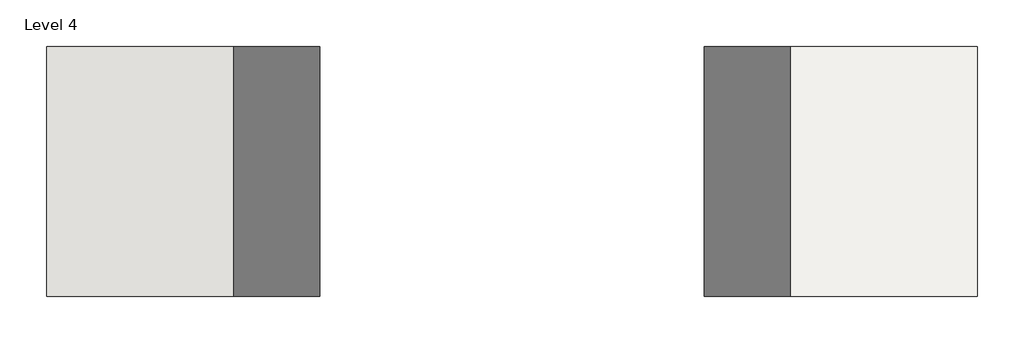
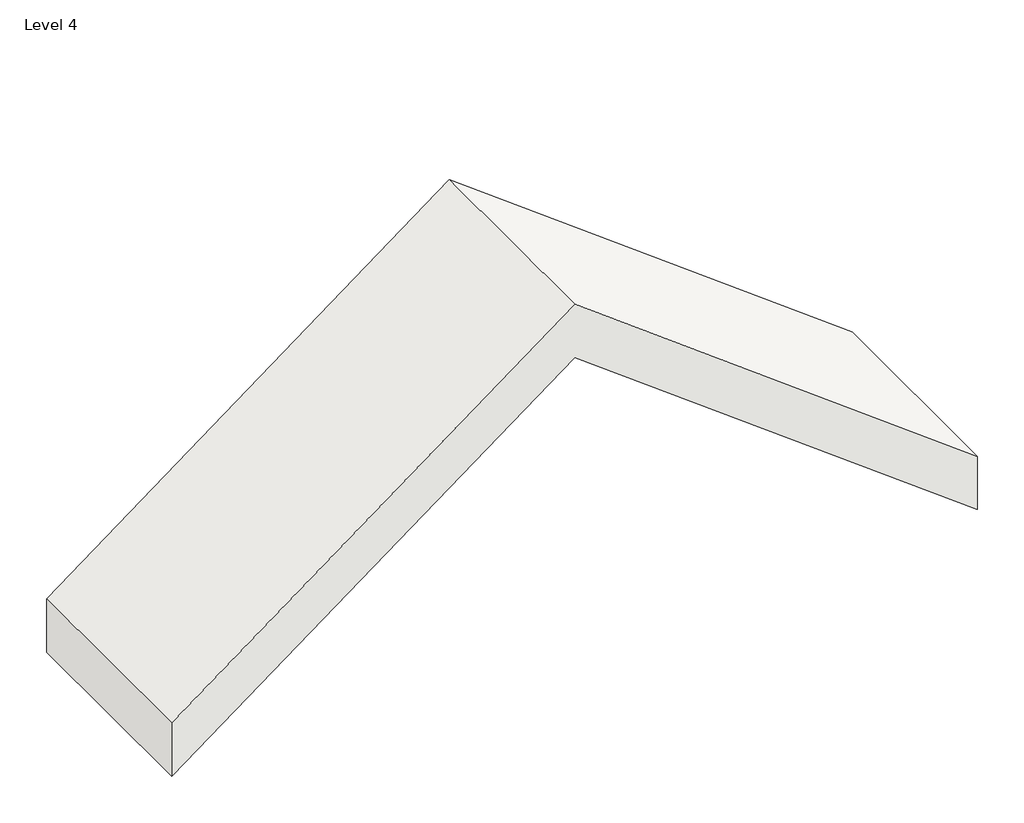
# One storey: 1 roof.
"""IFC4 building model written with IfcOpenShell, lengths in millimetres."""

from ifc_helpers import new_model, si_unit, frame, origin, place, context, project, spatial, polyline, outline, extrude, element, save

model = new_model("IFC4")

# Units and contexts
model_context = context("Model", 3, world=origin())
ifc_project = project(units=[si_unit("LENGTHUNIT", "METRE", prefix="MILLI")], contexts=[model_context])

# Site, building, storey
site = spatial("IfcSite", under=ifc_project)
building = spatial("IfcBuilding", under=site)
storey = spatial("IfcBuildingStorey", under=building, Name="Level 4", Elevation=9144.0)

# Roof
placement = place(None, origin())
element("IfcRoof", 1, ObjectType="Generic - 12\"", at=placement, inside=storey, context=model_context, shape_type="SweptSolid", body=[
    extrude(outline(polyline([(9525.0, -3625.114323), (11568.1125, -6349.264323), (9525.0, -9073.414323), (9144.0, -9073.414323), (11187.1125, -6349.264323), (9144.0, -3625.114323), (9525.0, -3625.114323)])), frame((0.0, -13864.3466243, 0.0), z_axis=(0.0, 1.0, 0.0), x_axis=(0.0, 0.0, 1.0)), (0.0, 0.0, 1.0), 1464.2950527),
])

save(model, "model.ifc")

# Revit data of these elements
# Type "Generic - 12\""
#   Assembly Code = "B1020"
#   Layers, outside or top first: 1' - 0" no material (function 1)
# Element 1 (IfcRoof, "Generic - 12\"")
#   built-in parameter 1001705 = 37.9531 (stored number, unit not read)
#   built-in parameter 1001710 = 33615
#   Phase Created = New Construction
#   Materials on its faces: "Default Roof"
# Materials
#   "Default Roof": colour RGB 88 101 114, transparency 0, Cost = 0
